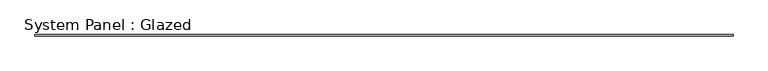
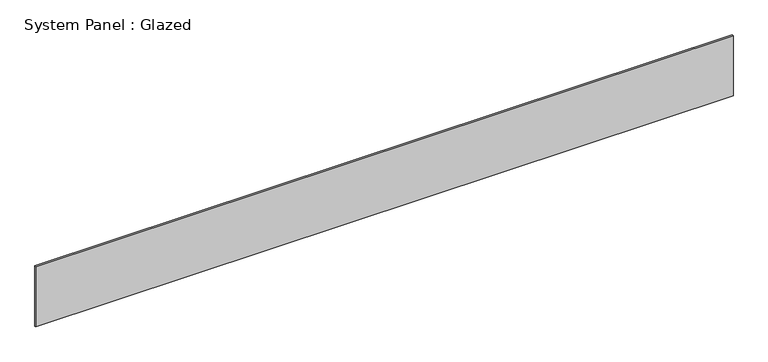
"""IFC4 building model written with IfcOpenShell, lengths in millimetres: plate geometry, System Panel : Glazed."""

from ifc_helpers import new_model, si_unit, origin, origin_with_axes, place, context, project, spatial, polyline, outline, extrude, source, transform, mapped, element, save


def system_panel_glazed_16aad0d4(model_context):
    return source(origin(), model_context, "Body", "SweptSolid", [
        extrude(outline(polyline([(6334.9276373, 19.05), (-6334.9276373, 19.05), (-6334.9276373, 44.45), (6334.9276373, 44.45), (6334.9276373, 19.05)])), origin_with_axes(), (0.0, 0.0, 1.0), 1155.7),
    ])


if __name__ == "__main__":
    model = new_model("IFC4")
    model_context = context("Model", 3, world=origin())
    ifc_project = project(units=[si_unit("LENGTHUNIT", "METRE", prefix="MILLI")], contexts=[model_context])
    site = spatial("IfcSite", under=ifc_project)
    building = spatial("IfcBuilding", under=site)
    placement = place(None, origin())
    system_panel_glazed_shape = system_panel_glazed_16aad0d4(model_context)
    element("IfcPlate", 1, ObjectType="System Panel : Glazed", at=placement, inside=building, context=model_context, shape_type="MappedRepresentation", body=[
        mapped(system_panel_glazed_shape, transform((0.0, 0.0, 0.0), x_axis=(1.0, 0.0, 0.0), y_axis=(0.0, 1.0, 0.0), z_axis=(0.0, 0.0, 1.0))),
    ])
    save(model, "model.ifc")

# Revit data of these elements
# Type "System Panel : Glazed"
#   Construction Type Id = "GSP4R"
#   Analytic Construction = "1/8 in Pilkington single glazing"
#   Visual Light Transmittance = 0.9
#   Solar Heat Gain Coefficient = 0.86
#   Heat Transfer Coefficient (U) = 1.18115 BTU/(h·ft²·°F)
# Element 1 (IfcPlate, "System Panel : Glazed")
#   Materials on its faces: "Glass"
# Materials
#   "Glass": class "Glass", colour RGB 0 128 192, transparency 0.75, Description = "Soda Lime Glass", Cost = 0
